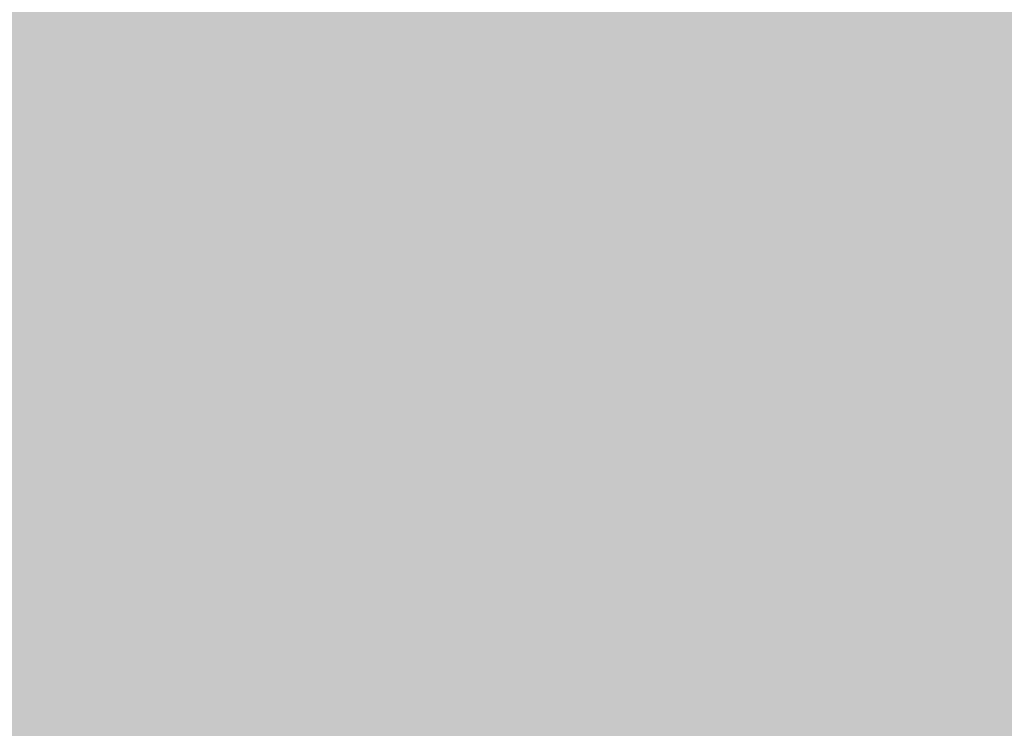
# Model space of a CAD drawing. Units: feet. Extents: x 3168 to 4724, y 827 to 1477.
# Tile 120 of 256: x 3298.68 to 3316.07, y 1074.89 to 1087.4. Entities that reach past the tile are written whole.
import ezdxf

# ---------------------------------------------------------------- set-up
doc = ezdxf.new("R2010")
doc.units = ezdxf.units.FT
doc.layers.add('A-ELEV-PATT', color=8, linetype='Continuous', lineweight=13)

msp = doc.modelspace()

# ---------------------------------------------------------------- hatches: boundary and pattern name
at = {"layer": 'A-ELEV-PATT'}
h = msp.add_hatch(color=256, dxfattribs=at)
h.dxf.hatch_style = 1
edge = h.paths.add_edge_path()
edge.add_ellipse((3552.906, 979.22), major_axis=(36.745, 0), ratio=0.484848, start_angle=0, end_angle=360)
edge = h.paths.add_edge_path()
edge.add_ellipse((3559.892, 929.252), major_axis=(36.745, 0), ratio=0.484848, start_angle=0, end_angle=360)
edge = h.paths.add_edge_path()
edge.add_line((3299.317, 1198.606), (3479.917, 1198.606))
edge.add_line((3479.917, 1198.606), (3479.917, 1209.869))
edge.add_spline(control_points=[(3479.917, 1209.869), (3464.301, 1209.869), (3448.686, 1209.869), (3410.949, 1209.869), (3388.828, 1209.869), (3355.647, 1209.869), (3344.586, 1209.869), (3327.996, 1209.869), (3322.466, 1209.869), (3314.17, 1209.869), (3311.405, 1209.869), (3307.257, 1209.869), (3305.875, 1209.869), (3303.801, 1209.869), (3303.11, 1209.869), (3302.073, 1209.869), (3301.727, 1209.869), (3301.209, 1209.869), (3301.036, 1209.869), (3300.777, 1209.869), (3300.69, 1209.869), (3300.561, 1209.869), (3300.517, 1209.869), (3300.453, 1209.869), (3300.431, 1209.869), (3300.399, 1209.869), (3300.388, 1209.869), (3300.366, 1209.869), (3300.346, 1209.869), (3300.346, 1209.869), (3300.346, 1209.869), (3300.343, 1209.869), (3300.341, 1209.869), (3300.338, 1209.869), (3300.337, 1209.869), (3300.334, 1209.869), (3300.332, 1209.869), (3300.326, 1209.869), (3300.321, 1209.869), (3300.311, 1209.869), (3300.306, 1209.869), (3300.291, 1209.869), (3300.28, 1209.869), (3300.232, 1209.869), (3300.195, 1209.869), (3299.951, 1209.871), (3299.745, 1209.874), (3299.437, 1209.883), (3299.334, 1209.887), (3299.181, 1209.893), (3299.13, 1209.895), (3298.652, 1209.917), (3298.229, 1209.946), (3297.602, 1210.002), (3297.393, 1210.023), (3297.083, 1210.058), (3296.979, 1210.07), (3296.293, 1210.155), (3295.718, 1210.243), (3294.869, 1210.399), (3294.588, 1210.454), (3294.169, 1210.543), (3294.03, 1210.574), (3291.707, 1211.101), (3289.654, 1211.813), (3285.776, 1213.564), (3283.951, 1214.603), (3280.512, 1216.98), (3278.897, 1218.318), (3276.38, 1220.829), (3275.416, 1221.918), (3274.039, 1223.708), (3273.581, 1224.35), (3273.143, 1225.016)], knot_values=[39.119033, 39.119033, 39.119033, 39.119033, 39.286353, 39.286353, 39.523379, 39.523379, 39.641892, 39.641892, 39.701148, 39.701148, 39.730777, 39.730777, 39.745591, 39.745591, 39.752998, 39.752998, 39.756701, 39.756701, 39.758553, 39.758553, 39.759479, 39.759479, 39.759942, 39.759942, 39.760173, 39.760173, 39.760289, 39.760289, 39.760405, 39.760405, 39.760463, 39.760463, 39.763389, 39.763389, 39.764851, 39.764851, 39.767304, 39.767304, 39.773825, 39.773825, 39.78057, 39.78057, 39.79477, 39.79477, 39.845194, 39.845194, 40.126715, 40.126715, 40.267476, 40.267476, 40.337856, 40.337856, 40.927023, 40.927023, 41.221606, 41.221606, 41.368898, 41.368898, 42.202622, 42.202622, 42.619485, 42.619485, 42.827916, 42.827916, 46.118323, 46.118323, 49.408731, 49.408731, 52.699139, 52.699139, 54.927489, 54.927489, 56.104228, 56.104228, 56.104228, 56.104228], weights=[1, 1, 1, 1, 1, 1, 1, 1, 1, 1, 1, 1, 1, 1, 1, 1, 1, 1, 1, 1, 1, 1, 1, 1, 1, 1, 1, 1, 1, 1, 1, 1, 1, 1, 1, 1, 1, 1, 1, 1, 1, 1, 1, 1, 1, 1, 1, 1, 1, 1, 1, 1, 1, 1, 1, 1, 1, 1, 1, 1, 1, 1, 1, 1, 1, 1, 1, 1, 1, 1, 1, 1, 1, 1], degree=3, periodic=0)
edge.add_line((3273.143, 1225.016), (3273.143, 1099.016))
edge.add_line((3273.143, 1099.016), (3299.317, 1099.016))
edge.add_line((3299.317, 1099.016), (3299.317, 1198.606))
edge = h.paths.add_edge_path()
edge.add_line((3304.758, 1324.158), (3479.917, 1324.158))
edge.add_line((3479.917, 1324.158), (3479.917, 1335.715))
edge.add_line((3479.917, 1335.715), (3269.162, 1335.715))
edge.add_spline(control_points=[(3269.162, 1335.715), (3264.024, 1335.715), (3258.364, 1328.958), (3259.264, 1323.9)], knot_values=[0, 0, 0, 0, 15.412191, 15.412191, 15.412191, 15.412191], degree=3, periodic=0)
edge.add_line((3259.264, 1323.9), (3265.517, 1288.769))
edge.add_line((3265.517, 1288.769), (3275.265, 1261.546))
edge.add_line((3275.265, 1261.546), (3304.758, 1261.546))
edge.add_line((3304.758, 1261.546), (3304.758, 1324.158))
h = msp.add_hatch(color=256, dxfattribs=at)
h.dxf.hatch_style = 1
h.paths.add_polyline_path([(3384.525, 1099.016), (3335.029, 1099.016), (3299.317, 1099.016), (3273.143, 1099.016), (3217.565, 1099.016), (3168.069, 827.116), (3335.029, 827.116)])

doc.saveas('drawing.dxf')
